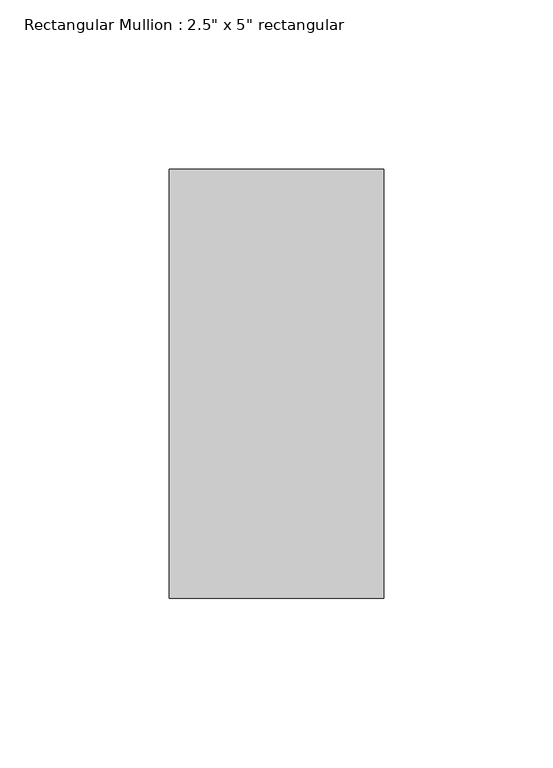
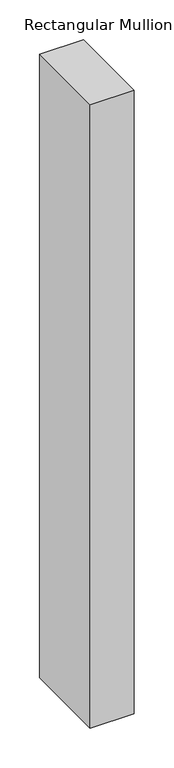
"""IFC4 building model written with IfcOpenShell, lengths in millimetres: member geometry."""

from ifc_helpers import new_model, si_unit, frame, origin, place, context, project, spatial, polyline, outline, extrude, source, transform, mapped, element, save


def member_57aae9a7(model_context):
    return source(origin(), model_context, "Body", "SweptSolid", [
        extrude(outline(polyline([(0.0, 63.5), (0.0, -63.5), (-63.5, -63.5), (-63.5, 63.5), (0.0, 63.5)])), frame((0.0, 0.0, -954.6166667), z_axis=(0.0, 0.0, 1.0), x_axis=(1.0, 0.0, 0.0)), (0.0, 0.0, 1.0), 954.6166667),
    ])


if __name__ == "__main__":
    model = new_model("IFC4")
    model_context = context("Model", 3, world=origin())
    ifc_project = project(units=[si_unit("LENGTHUNIT", "METRE", prefix="MILLI")], contexts=[model_context])
    site = spatial("IfcSite", under=ifc_project)
    building = spatial("IfcBuilding", under=site)
    placement = place(None, origin())
    member_shape = member_57aae9a7(model_context)
    element("IfcMember", 1, ObjectType="Rectangular Mullion : 2.5\" x 5\" rectangular", at=placement, inside=building, context=model_context, shape_type="MappedRepresentation", body=[
        mapped(member_shape, transform((0.0, 0.0, 0.0), x_axis=(1.0, 0.0, 0.0), y_axis=(0.0, 1.0, 0.0), z_axis=(0.0, 0.0, 1.0))),
    ])
    save(model, "model.ifc")

# Revit data of these elements
# Type "Rectangular Mullion : 2.5\" x 5\" rectangular"
#   built-in parameter 1007304 = 0.416667 (stored number, unit not read)
#   built-in parameter 1007301 = 0.104167 (stored number, unit not read)
#   built-in parameter 1007300 = 0.104167 (stored number, unit not read)
# Element 1 (IfcMember, "Rectangular Mullion : 2.5\" x 5\" rectangular")
#   Materials on its faces: "Aluminum"
# Materials
#   "Aluminum": class "Metal", colour RGB 247 247 247, transparency 0, Description = "Aluminum 6061", Cost = 0
